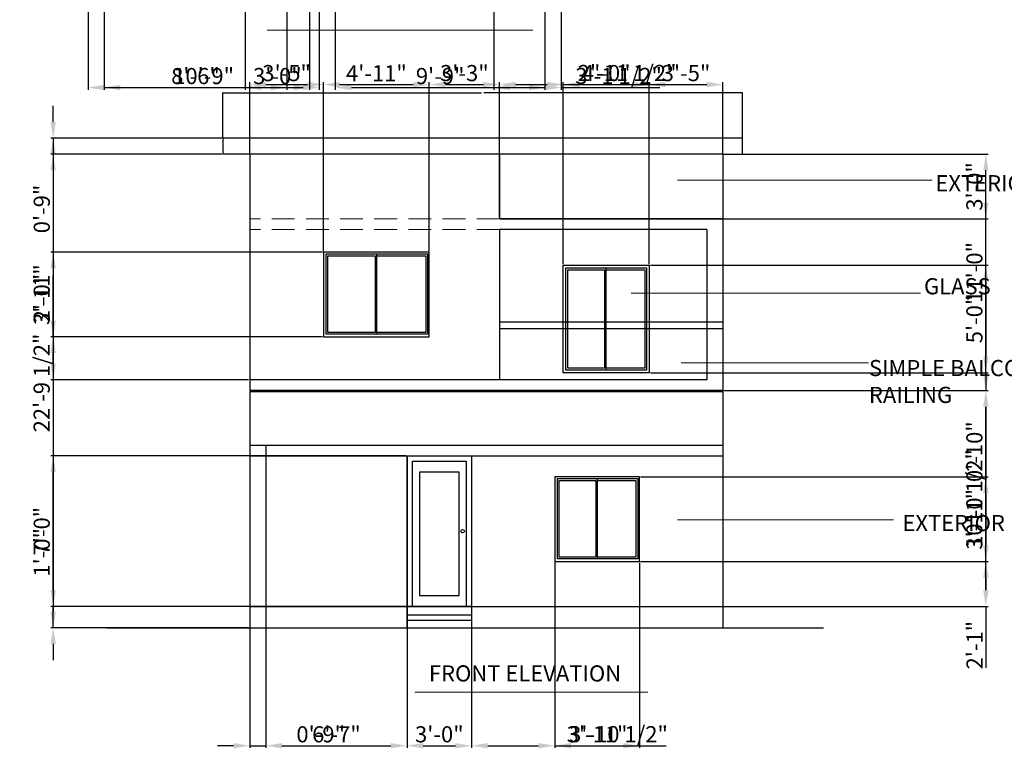
# Model space of a CAD drawing. Units: inches. Extents: x 2429 to 3343, y 1496 to 2530.
# Tile 1 of 7: x 2442 to 2991, y 1496 to 1910. Entities that reach past the tile are written whole.
import ezdxf

# ---------------------------------------------------------------- set-up
doc = ezdxf.new("R2010")
doc.units = ezdxf.units.IN
doc.linetypes.add('DASHED', pattern=[19.05, 12.7, -6.35])
for name, color, linetype, lineweight in [('A-ANNO-DIMS', 2, 'Continuous', 18), ('A-ANNO-TEXT', 7, 'Continuous', 18), ('A-ELEV', 7, 'Continuous', 25), ('A-ELEV-OVHD', 8, 'DASHED', 18)]:
    doc.layers.add(name, color=color, linetype=linetype, lineweight=lineweight)
doc.styles.get("Standard").update_dxf_attribs({"font": 'arial.ttf'})
doc.dimstyles.new('ISO-25', dxfattribs={"dimtxt": 9, "dimasz": 9, "dimexe": 1.25, "dimexo": 0.625, "dimtad": 1, "dimdec": 1, "dimlunit": 3, "dimtxsty": 'Standard', "dimcen": 9, "dimadec": 0, "dimazin": 0, "dimtfac": 1, "dimtdec": 1, "dimtmove": 0, "dimatfit": 3, "dimfxl": 1, "dimarcsym": 0})
doc.dimstyles.get("Standard").update_dxf_attribs({"dimtxt": 0.18, "dimasz": 0.18, "dimexe": 0.18, "dimexo": 0.0625, "dimgap": 0.09, "dimtad": 0, "dimtih": 1, "dimtoh": 1, "dimdec": 4, "dimzin": 0, "dimdsep": 46, "dimtxsty": 'Standard', "dimcen": 0.09, "dimadec": 0, "dimazin": 0, "dimtfac": 1, "dimtdec": 4, "dimtofl": 0, "dimtmove": 0, "dimatfit": 3, "dimfxl": 1, "dimtolj": 1, "dimtzin": 0, "dimarcsym": 0})

# ---------------------------------------------------------------- blocks, each defined once
blk = doc.blocks.new('*U18')
blk.add_lwpolyline([(3.12, 0.01), (0.12, 0.01), (0.12, 84.01), (36.12, 84.01), (36.12, 0.01), (33.12, 0.01)])
for points in [[(33.12, 80.99), (33.12, 0.01), (3.12, 0.01), (3.12, 80.99)], [(29.12, 6.01), (29.12, 74.99), (7.12, 74.99), (7.12, 6.01)]]:
    blk.add_lwpolyline(points, close=True)
blk.add_circle((31.12, 42.01), 1)
blk = doc.blocks.new('*U15')
for p, q in [((38.1, 38.1), (38.1, 1176.3)), ((38.1, 1176.3), (607.2, 1176.3)), ((607.2, 38.1), (607.2, 1176.3)), ((607.2, 1176.3), (1176.3, 1176.3)), ((1176.3, 1176.3), (1176.3, 38.1)), ((607.2, 38.1), (38.1, 38.1)), ((1176.3, 38.1), (607.2, 38.1))]:
    blk.add_line(p, q)
blk.add_lwpolyline([(0, 0), (1200, 0), (1200, 1200), (0, 1200)], close=True)
for points in [[(581.8, 1150.9), (581.8, 63.5), (63.5, 63.5), (63.5, 1150.9), (581.8, 1150.9)], [(607.2, 1150.9), (1150.9, 1150.9), (1150.9, 63.5), (607.2, 63.5)]]:
    blk.add_lwpolyline(points)
blk = doc.blocks.new('*U20')
for p, q in [((1.5, 1.5), (1.5, 58.5)), ((1.5, 58.5), (24, 58.5)), ((24, 1.5), (24, 58.5)), ((24, 58.5), (46.5, 58.5)), ((46.5, 58.5), (46.5, 1.5)), ((24, 1.5), (1.5, 1.5)), ((46.5, 1.5), (24, 1.5))]:
    blk.add_line(p, q)
blk.add_lwpolyline([(0, 0), (0, 60), (48, 60), (48, 0)], close=True)
for points in [[(23, 57.5), (23, 2.5), (2.5, 2.5), (2.5, 57.5), (23, 57.5)], [(24, 57.5), (45.5, 57.5), (45.5, 2.5), (24, 2.5)]]:
    blk.add_lwpolyline(points)
blk = doc.blocks.new('*U21')
for p, q in [((38.1, 38.1), (38.1, 1176.3)), ((38.1, 1176.3), (757.2, 1176.3)), ((757.2, 38.1), (757.2, 1176.3)), ((757.2, 1176.3), (1476.3, 1176.3)), ((1476.3, 1176.3), (1476.3, 38.1)), ((757.2, 38.1), (38.1, 38.1)), ((1476.3, 38.1), (757.2, 38.1))]:
    blk.add_line(p, q)
blk.add_lwpolyline([(0, 0), (1500, 0), (1500, 1200), (0, 1200)], close=True)
for points in [[(731.8, 1150.9), (731.8, 63.5), (63.5, 63.5), (63.5, 1150.9), (731.8, 1150.9)], [(757.2, 1150.9), (1450.9, 1150.9), (1450.9, 63.5), (757.2, 63.5)]]:
    blk.add_lwpolyline(points)
blk = doc.blocks.new('*D22')
at = {"layer": 'A-ANNO-DIMS', "color": 0, "lineweight": -2, "transparency": 16777216}
for p, q in [((2554.96, 1843.52), (2554.96, 1868.85)), ((2555.14, 1868.67), (2699.36, 1868.67)), ((2844.78, 1868.67), (2700.57, 1868.67)), ((2844.96, 1843.52), (2844.96, 1868.85))]:
    blk.add_line(p, q, dxfattribs=at)
at = {"layer": 'A-ANNO-DIMS', "color": 0, "transparency": 16777216}
for points in [[(2555.14, 1868.7), (2555.14, 1868.64), (2554.96, 1868.67)], [(2844.78, 1868.7), (2844.78, 1868.64), (2844.96, 1868.67)]]:
    blk.add_solid(points, dxfattribs=at)
at = {"layer": 'Defpoints', "color": 0, "transparency": 16777216}
for p in [(2844.96, 1868.67), (2554.96, 1843.46), (2844.96, 1843.46)]:
    blk.add_point(p, dxfattribs=at)
at = {"layer": 'A-ANNO-DIMS', "color": 0, "transparency": 16777216, "insert": (2699.96, 1868.67), "char_height": 0.18, "attachment_point": 5}
blk.add_mtext('\\A1;290.0000', dxfattribs=at)
blk = doc.blocks.new('*D34')
at = {"layer": 'A-ANNO-DIMS', "color": 0, "lineweight": -2, "transparency": 16777216}
for p, q in [((2590.68, 2320.13), (2590.68, 1870.45)), ((2488.77, 2248.13), (2488.77, 1870.45)), ((2497.77, 1871.7), (2581.68, 1871.7))]:
    blk.add_line(p, q, dxfattribs=at)
at = {"layer": 'A-ANNO-DIMS', "color": 0, "transparency": 16777216}
for points in [[(2497.77, 1873.2), (2497.77, 1870.2), (2488.77, 1871.7)], [(2581.68, 1873.2), (2581.68, 1870.2), (2590.68, 1871.7)]]:
    blk.add_solid(points, dxfattribs=at)
at = {"layer": 'Defpoints', "color": 0, "transparency": 16777216}
for p in [(2590.68, 2320.75), (2488.77, 2248.75), (2590.68, 1871.7)]:
    blk.add_point(p, dxfattribs=at)
at = {"layer": 'A-ANNO-DIMS', "color": 0, "transparency": 16777216, "insert": (2539.73, 1876.92), "char_height": 9, "attachment_point": 5}
blk.add_mtext('8\'-6"', dxfattribs=at)
blk = doc.blocks.new('*D38')
at = {"layer": 'A-ANNO-DIMS', "color": 0, "lineweight": -2, "transparency": 16777216}
for p, q in [((2617.77, 2011.13), (2617.77, 1870.45)), ((2734.77, 2011.13), (2734.77, 1870.45)), ((2626.77, 1871.7), (2725.77, 1871.7))]:
    blk.add_line(p, q, dxfattribs=at)
at = {"layer": 'A-ANNO-DIMS', "color": 0, "transparency": 16777216}
for points in [[(2626.77, 1873.2), (2626.77, 1870.2), (2617.77, 1871.7)], [(2725.77, 1873.2), (2725.77, 1870.2), (2734.77, 1871.7)]]:
    blk.add_solid(points, dxfattribs=at)
at = {"layer": 'Defpoints', "color": 0, "transparency": 16777216}
for p in [(2617.77, 2011.75), (2734.77, 2011.75), (2734.77, 1871.7)]:
    blk.add_point(p, dxfattribs=at)
at = {"layer": 'A-ANNO-DIMS', "color": 0, "transparency": 16777216, "insert": (2676.27, 1876.92), "char_height": 9, "attachment_point": 5}
blk.add_mtext('9\'-9"', dxfattribs=at)
blk = doc.blocks.new('*D44')
at = {"layer": 'A-ANNO-DIMS', "color": 0, "lineweight": -2, "transparency": 16777216}
for p, q in [((2608.77, 2002.13), (2608.77, 1870.45)), ((2479.77, 1970.81), (2479.77, 1870.45)), ((2488.77, 1871.7), (2599.77, 1871.7))]:
    blk.add_line(p, q, dxfattribs=at)
at = {"layer": 'A-ANNO-DIMS', "color": 0, "transparency": 16777216}
for points in [[(2488.77, 1873.2), (2488.77, 1870.2), (2479.77, 1871.7)], [(2599.77, 1873.2), (2599.77, 1870.2), (2608.77, 1871.7)]]:
    blk.add_solid(points, dxfattribs=at)
at = {"layer": 'Defpoints', "color": 0, "transparency": 16777216}
for p in [(2608.77, 2002.75), (2479.77, 1971.44), (2608.77, 1871.7)]:
    blk.add_point(p, dxfattribs=at)
at = {"layer": 'A-ANNO-DIMS', "color": 0, "transparency": 16777216, "insert": (2544.27, 1876.92), "char_height": 9, "attachment_point": 5}
blk.add_mtext('10\'-9"', dxfattribs=at)
blk = doc.blocks.new('*D45')
at = {"layer": 'A-ANNO-DIMS', "color": 0, "lineweight": -2, "transparency": 16777216}
for p, q in [((2567.44, 2072.42), (2567.44, 1870.45)), ((2603.44, 2071.13), (2603.44, 1870.45)), ((2576.44, 1871.7), (2594.44, 1871.7))]:
    blk.add_line(p, q, dxfattribs=at)
at = {"layer": 'A-ANNO-DIMS', "color": 0, "transparency": 16777216}
for points in [[(2576.44, 1873.2), (2576.44, 1870.2), (2567.44, 1871.7)], [(2594.44, 1873.2), (2594.44, 1870.2), (2603.44, 1871.7)]]:
    blk.add_solid(points, dxfattribs=at)
at = {"layer": 'Defpoints', "color": 0, "transparency": 16777216}
for p in [(2567.44, 2073.04), (2603.44, 2071.75), (2603.44, 1871.7)]:
    blk.add_point(p, dxfattribs=at)
at = {"layer": 'A-ANNO-DIMS', "color": 0, "transparency": 16777216, "insert": (2585.44, 1876.92), "char_height": 9, "attachment_point": 5}
blk.add_mtext('3\'-0"', dxfattribs=at)
blk = doc.blocks.new('*D55')
at = {"layer": 'A-ANNO-DIMS', "color": 0, "lineweight": -2, "transparency": 16777216}
for p, q in [((2706.27, 2002.13), (2706.27, 1870.45)), ((2743.77, 2002.13), (2743.77, 1870.45)), ((2715.27, 1871.7), (2734.77, 1871.7)), ((2743.77, 1871.7), (2798.91, 1871.7))]:
    blk.add_line(p, q, dxfattribs=at)
at = {"layer": 'A-ANNO-DIMS', "color": 0, "transparency": 16777216}
for points in [[(2715.27, 1873.2), (2715.27, 1870.2), (2706.27, 1871.7)], [(2734.77, 1873.2), (2734.77, 1870.2), (2743.77, 1871.7)]]:
    blk.add_solid(points, dxfattribs=at)
at = {"layer": 'Defpoints', "color": 0, "transparency": 16777216}
for p in [(2706.27, 2002.75), (2743.77, 2002.75), (2743.77, 1871.7)]:
    blk.add_point(p, dxfattribs=at)
at = {"layer": 'A-ANNO-DIMS', "color": 0, "transparency": 16777216, "insert": (2775.84, 1876.98), "char_height": 9, "attachment_point": 5}
blk.add_mtext('3\'-1 1/2"', dxfattribs=at)
blk = doc.blocks.new('*D84')
at = {"layer": 'A-ANNO-DIMS', "color": 0, "lineweight": -2, "transparency": 16777216}
for p, q in [((2554.34, 1843.46), (2459.08, 1843.46)), ((2460.33, 1834.46), (2460.33, 1579)), ((2569.38, 1570), (2459.08, 1570))]:
    blk.add_line(p, q, dxfattribs=at)
at = {"layer": 'A-ANNO-DIMS', "color": 0, "transparency": 16777216}
for points in [[(2458.83, 1834.46), (2461.83, 1834.46), (2460.33, 1843.46)], [(2458.83, 1579), (2461.83, 1579), (2460.33, 1570)]]:
    blk.add_solid(points, dxfattribs=at)
at = {"layer": 'Defpoints', "color": 0, "transparency": 16777216}
for p in [(2554.96, 1843.46), (2460.33, 1570), (2570, 1570)]:
    blk.add_point(p, dxfattribs=at)
at = {"layer": 'A-ANNO-DIMS', "color": 0, "transparency": 16777216, "insert": (2455.05, 1706.73), "char_height": 9, "attachment_point": 5, "rotation": 90}
blk.add_mtext('22\'-9 1/2"', dxfattribs=at)
blk = doc.blocks.new('*D85')
at = {"layer": 'A-ANNO-DIMS', "color": 0, "lineweight": -2, "transparency": 16777216}
for p, q in [((2460.33, 1852.46), (2460.33, 1861.46)), ((2554.34, 1843.46), (2459.08, 1843.46)), ((2460.33, 1843.46), (2460.33, 1834.46)), ((2554.34, 1834.46), (2459.08, 1834.46)), ((2460.33, 1825.46), (2460.33, 1791.28))]:
    blk.add_line(p, q, dxfattribs=at)
at = {"layer": 'A-ANNO-DIMS', "color": 0, "transparency": 16777216}
for points in [[(2458.83, 1852.46), (2461.83, 1852.46), (2460.33, 1843.46)], [(2458.83, 1825.46), (2461.83, 1825.46), (2460.33, 1834.46)]]:
    blk.add_solid(points, dxfattribs=at)
at = {"layer": 'Defpoints', "color": 0, "transparency": 16777216}
for p in [(2554.96, 1843.46), (2460.33, 1834.46), (2554.96, 1834.46)]:
    blk.add_point(p, dxfattribs=at)
at = {"layer": 'A-ANNO-DIMS', "color": 0, "transparency": 16777216, "insert": (2455.11, 1803.87), "char_height": 9, "attachment_point": 5, "rotation": 90}
blk.add_mtext('0\'-9"', dxfattribs=at)
blk = doc.blocks.new('*D86')
at = {"layer": 'A-ANNO-DIMS', "color": 0, "lineweight": -2, "transparency": 16777216}
for p, q in [((2460.33, 1591), (2460.33, 1624.33)), ((2569.38, 1582), (2459.08, 1582)), ((2460.33, 1570), (2460.33, 1582)), ((2569.38, 1570), (2459.08, 1570)), ((2460.33, 1561), (2460.33, 1552))]:
    blk.add_line(p, q, dxfattribs=at)
at = {"layer": 'A-ANNO-DIMS', "color": 0, "transparency": 16777216}
for points in [[(2458.83, 1591), (2461.83, 1591), (2460.33, 1582)], [(2458.83, 1561), (2461.83, 1561), (2460.33, 1570)]]:
    blk.add_solid(points, dxfattribs=at)
at = {"layer": 'Defpoints', "color": 0, "transparency": 16777216}
for p in [(2460.33, 1582), (2570, 1582), (2570, 1570)]:
    blk.add_point(p, dxfattribs=at)
at = {"layer": 'A-ANNO-DIMS', "color": 0, "transparency": 16777216, "insert": (2455.11, 1612.16), "char_height": 9, "attachment_point": 5, "rotation": 90}
blk.add_mtext('1\'-0"', dxfattribs=at)
blk = doc.blocks.new('*D87')
at = {"layer": 'A-ANNO-DIMS', "color": 0, "lineweight": -2, "transparency": 16777216}
for p, q in [((2834.63, 1702.46), (2982.04, 1702.46)), ((2980.79, 1591), (2980.79, 1693.46)), ((2834.63, 1582), (2982.04, 1582))]:
    blk.add_line(p, q, dxfattribs=at)
at = {"layer": 'A-ANNO-DIMS', "color": 0, "transparency": 16777216}
for points in [[(2979.29, 1693.46), (2982.29, 1693.46), (2980.79, 1702.46)], [(2979.29, 1591), (2982.29, 1591), (2980.79, 1582)]]:
    blk.add_solid(points, dxfattribs=at)
at = {"layer": 'Defpoints', "color": 0, "transparency": 16777216}
for p in [(2834.01, 1702.46), (2980.79, 1702.46), (2834, 1582)]:
    blk.add_point(p, dxfattribs=at)
at = {"layer": 'A-ANNO-DIMS', "color": 0, "transparency": 16777216, "insert": (2975.51, 1642.23), "char_height": 9, "attachment_point": 5, "rotation": 90}
blk.add_mtext('10\'-0 1/2"', dxfattribs=at)
blk = doc.blocks.new('*D88')
at = {"layer": 'A-ANNO-DIMS', "color": 0, "lineweight": -2, "transparency": 16777216}
for p, q in [((2834.63, 1834.46), (2982.04, 1834.46)), ((2980.79, 1711.46), (2980.79, 1825.46)), ((2834.63, 1702.46), (2982.04, 1702.46))]:
    blk.add_line(p, q, dxfattribs=at)
at = {"layer": 'A-ANNO-DIMS', "color": 0, "transparency": 16777216}
for points in [[(2979.29, 1825.46), (2982.29, 1825.46), (2980.79, 1834.46)], [(2979.29, 1711.46), (2982.29, 1711.46), (2980.79, 1702.46)]]:
    blk.add_solid(points, dxfattribs=at)
at = {"layer": 'Defpoints', "color": 0, "transparency": 16777216}
for p in [(2834.01, 1834.46), (2980.79, 1834.46), (2834.01, 1702.46)]:
    blk.add_point(p, dxfattribs=at)
at = {"layer": 'A-ANNO-DIMS', "color": 0, "transparency": 16777216, "insert": (2975.57, 1768.46), "char_height": 9, "attachment_point": 5, "rotation": 90}
blk.add_mtext('11\'-0"', dxfattribs=at)
blk = doc.blocks.new('*D89')
at = {"layer": 'A-ANNO-DIMS', "color": 0, "lineweight": -2, "transparency": 16777216}
for p, q in [((2570.01, 1835.08), (2570.01, 1874.61)), ((2611.16, 1780.33), (2611.16, 1874.61)), ((2579.01, 1873.36), (2602.16, 1873.36))]:
    blk.add_line(p, q, dxfattribs=at)
at = {"layer": 'A-ANNO-DIMS', "color": 0, "transparency": 16777216}
for points in [[(2579.01, 1874.86), (2579.01, 1871.86), (2570.01, 1873.36)], [(2602.16, 1874.86), (2602.16, 1871.86), (2611.16, 1873.36)]]:
    blk.add_solid(points, dxfattribs=at)
at = {"layer": 'Defpoints', "color": 0, "transparency": 16777216}
for p in [(2611.16, 1873.36), (2570.01, 1834.46), (2611.16, 1779.7)]:
    blk.add_point(p, dxfattribs=at)
at = {"layer": 'A-ANNO-DIMS', "color": 0, "transparency": 16777216, "insert": (2590.58, 1878.58), "char_height": 9, "attachment_point": 5}
blk.add_mtext('3\'-5"', dxfattribs=at)
blk = doc.blocks.new('*D90')
at = {"layer": 'A-ANNO-DIMS', "color": 0, "lineweight": -2, "transparency": 16777216}
for p, q in [((2611.16, 1780.33), (2611.16, 1874.61)), ((2670.21, 1780.33), (2670.21, 1874.61)), ((2620.16, 1873.36), (2661.21, 1873.36))]:
    blk.add_line(p, q, dxfattribs=at)
at = {"layer": 'A-ANNO-DIMS', "color": 0, "transparency": 16777216}
for points in [[(2620.16, 1874.86), (2620.16, 1871.86), (2611.16, 1873.36)], [(2661.21, 1874.86), (2661.21, 1871.86), (2670.21, 1873.36)]]:
    blk.add_solid(points, dxfattribs=at)
at = {"layer": 'Defpoints', "color": 0, "transparency": 16777216}
for p in [(2670.21, 1873.36), (2611.16, 1779.7), (2670.21, 1779.7)]:
    blk.add_point(p, dxfattribs=at)
at = {"layer": 'A-ANNO-DIMS', "color": 0, "transparency": 16777216, "insert": (2640.69, 1878.5), "char_height": 9, "attachment_point": 5}
blk.add_mtext('4\'-11"', dxfattribs=at)
blk = doc.blocks.new('*D91')
at = {"layer": 'A-ANNO-DIMS', "color": 0, "lineweight": -2, "transparency": 16777216}
for p, q in [((2670.21, 1780.33), (2670.21, 1874.61)), ((2709.37, 1799.08), (2709.37, 1874.61)), ((2679.21, 1873.36), (2700.37, 1873.36))]:
    blk.add_line(p, q, dxfattribs=at)
at = {"layer": 'A-ANNO-DIMS', "color": 0, "transparency": 16777216}
for points in [[(2679.21, 1874.86), (2679.21, 1871.86), (2670.21, 1873.36)], [(2700.37, 1874.86), (2700.37, 1871.86), (2709.37, 1873.36)]]:
    blk.add_solid(points, dxfattribs=at)
at = {"layer": 'Defpoints', "color": 0, "transparency": 16777216}
for p in [(2709.37, 1873.36), (2709.37, 1798.46), (2670.21, 1779.7)]:
    blk.add_point(p, dxfattribs=at)
at = {"layer": 'A-ANNO-DIMS', "color": 0, "transparency": 16777216, "insert": (2689.79, 1878.58), "char_height": 9, "attachment_point": 5}
blk.add_mtext('3\'-3"', dxfattribs=at)
blk = doc.blocks.new('*D92')
at = {"layer": 'A-ANNO-DIMS', "color": 0, "lineweight": -2, "transparency": 16777216}
for p, q in [((2709.37, 1799.08), (2709.37, 1874.61)), ((2744.96, 1773.08), (2744.96, 1874.61)), ((2718.37, 1873.36), (2735.96, 1873.36)), ((2744.96, 1873.36), (2807.25, 1873.36))]:
    blk.add_line(p, q, dxfattribs=at)
at = {"layer": 'A-ANNO-DIMS', "color": 0, "transparency": 16777216}
for points in [[(2718.37, 1874.86), (2718.37, 1871.86), (2709.37, 1873.36)], [(2735.96, 1874.86), (2735.96, 1871.86), (2744.96, 1873.36)]]:
    blk.add_solid(points, dxfattribs=at)
at = {"layer": 'Defpoints', "color": 0, "transparency": 16777216}
for p in [(2744.96, 1873.36), (2709.37, 1798.46), (2744.96, 1772.46)]:
    blk.add_point(p, dxfattribs=at)
at = {"layer": 'A-ANNO-DIMS', "color": 0, "transparency": 16777216, "insert": (2780.61, 1878.64), "char_height": 9, "attachment_point": 5}
blk.add_mtext('2\'-11 1/2"', dxfattribs=at)
blk = doc.blocks.new('*D93')
at = {"layer": 'A-ANNO-DIMS', "color": 0, "lineweight": -2, "transparency": 16777216}
for p, q in [((2744.96, 1773.08), (2744.96, 1874.61)), ((2792.96, 1773.08), (2792.96, 1874.61)), ((2753.96, 1873.36), (2783.96, 1873.36))]:
    blk.add_line(p, q, dxfattribs=at)
at = {"layer": 'A-ANNO-DIMS', "color": 0, "transparency": 16777216}
for points in [[(2753.96, 1874.86), (2753.96, 1871.86), (2744.96, 1873.36)], [(2783.96, 1874.86), (2783.96, 1871.86), (2792.96, 1873.36)]]:
    blk.add_solid(points, dxfattribs=at)
at = {"layer": 'Defpoints', "color": 0, "transparency": 16777216}
for p in [(2792.96, 1873.36), (2744.96, 1772.46), (2792.96, 1772.46)]:
    blk.add_point(p, dxfattribs=at)
at = {"layer": 'A-ANNO-DIMS', "color": 0, "transparency": 16777216, "insert": (2768.96, 1878.58), "char_height": 9, "attachment_point": 5}
blk.add_mtext('4\'-0"', dxfattribs=at)
blk = doc.blocks.new('*D94')
at = {"layer": 'A-ANNO-DIMS', "color": 0, "lineweight": -2, "transparency": 16777216}
for p, q in [((2792.96, 1773.08), (2792.96, 1874.61)), ((2834.01, 1835.08), (2834.01, 1874.61)), ((2801.96, 1873.36), (2825.01, 1873.36))]:
    blk.add_line(p, q, dxfattribs=at)
at = {"layer": 'A-ANNO-DIMS', "color": 0, "transparency": 16777216}
for points in [[(2801.96, 1874.86), (2801.96, 1871.86), (2792.96, 1873.36)], [(2825.01, 1874.86), (2825.01, 1871.86), (2834.01, 1873.36)]]:
    blk.add_solid(points, dxfattribs=at)
at = {"layer": 'Defpoints', "color": 0, "transparency": 16777216}
for p in [(2834.01, 1873.36), (2834.01, 1834.46), (2792.96, 1772.46)]:
    blk.add_point(p, dxfattribs=at)
at = {"layer": 'A-ANNO-DIMS', "color": 0, "transparency": 16777216, "insert": (2813.48, 1878.58), "char_height": 9, "attachment_point": 5}
blk.add_mtext('3\'-5"', dxfattribs=at)
blk = doc.blocks.new('*D95')
at = {"layer": 'A-ANNO-DIMS', "color": 0, "lineweight": -2, "transparency": 16777216}
for p, q in [((2579, 1671.38), (2579, 1502.93)), ((2657.8, 1665.38), (2657.8, 1502.93)), ((2588, 1504.18), (2648.8, 1504.18))]:
    blk.add_line(p, q, dxfattribs=at)
at = {"layer": 'A-ANNO-DIMS', "color": 0, "transparency": 16777216}
for points in [[(2588, 1505.68), (2588, 1502.68), (2579, 1504.18)], [(2648.8, 1505.68), (2648.8, 1502.68), (2657.8, 1504.18)]]:
    blk.add_solid(points, dxfattribs=at)
at = {"layer": 'Defpoints', "color": 0, "transparency": 16777216}
for p in [(2579, 1672), (2657.8, 1666), (2657.8, 1504.18)]:
    blk.add_point(p, dxfattribs=at)
at = {"layer": 'A-ANNO-DIMS', "color": 0, "transparency": 16777216, "insert": (2618.4, 1509.4), "char_height": 9, "attachment_point": 5}
blk.add_mtext('6\'-7"', dxfattribs=at)
blk = doc.blocks.new('*D96')
at = {"layer": 'A-ANNO-DIMS', "color": 0, "lineweight": -2, "transparency": 16777216}
for p, q in [((2570, 1671.38), (2570, 1502.93)), ((2579, 1671.38), (2579, 1502.93)), ((2561, 1504.18), (2552, 1504.18)), ((2570, 1504.18), (2579, 1504.18)), ((2588, 1504.18), (2622.17, 1504.18))]:
    blk.add_line(p, q, dxfattribs=at)
at = {"layer": 'A-ANNO-DIMS', "color": 0, "transparency": 16777216}
for points in [[(2561, 1505.68), (2561, 1502.68), (2570, 1504.18)], [(2588, 1505.68), (2588, 1502.68), (2579, 1504.18)]]:
    blk.add_solid(points, dxfattribs=at)
at = {"layer": 'Defpoints', "color": 0, "transparency": 16777216}
for p in [(2570, 1672), (2579, 1672), (2579, 1504.18)]:
    blk.add_point(p, dxfattribs=at)
at = {"layer": 'A-ANNO-DIMS', "color": 0, "transparency": 16777216, "insert": (2609.59, 1509.4), "char_height": 9, "attachment_point": 5}
blk.add_mtext('0\'-9"', dxfattribs=at)
blk = doc.blocks.new('*D97')
at = {"layer": 'A-ANNO-DIMS', "color": 0, "lineweight": -2, "transparency": 16777216}
for p, q in [((2657.8, 1581.38), (2657.8, 1502.93)), ((2693.8, 1581.38), (2693.8, 1502.93)), ((2666.8, 1504.18), (2684.8, 1504.18))]:
    blk.add_line(p, q, dxfattribs=at)
at = {"layer": 'A-ANNO-DIMS', "color": 0, "transparency": 16777216}
for points in [[(2666.8, 1505.68), (2666.8, 1502.68), (2657.8, 1504.18)], [(2684.8, 1505.68), (2684.8, 1502.68), (2693.8, 1504.18)]]:
    blk.add_solid(points, dxfattribs=at)
at = {"layer": 'Defpoints', "color": 0, "transparency": 16777216}
for p in [(2657.8, 1582), (2693.8, 1582), (2693.8, 1504.18)]:
    blk.add_point(p, dxfattribs=at)
at = {"layer": 'A-ANNO-DIMS', "color": 0, "transparency": 16777216, "insert": (2675.8, 1509.4), "char_height": 9, "attachment_point": 5}
blk.add_mtext('3\'-0"', dxfattribs=at)
blk = doc.blocks.new('*D98')
at = {"layer": 'A-ANNO-DIMS', "color": 0, "lineweight": -2, "transparency": 16777216}
for p, q in [((2693.8, 1665.38), (2693.8, 1502.93)), ((2740.23, 1653.63), (2740.23, 1502.93)), ((2702.8, 1504.18), (2731.23, 1504.18)), ((2740.23, 1504.18), (2802.36, 1504.18))]:
    blk.add_line(p, q, dxfattribs=at)
at = {"layer": 'A-ANNO-DIMS', "color": 0, "transparency": 16777216}
for points in [[(2702.8, 1505.68), (2702.8, 1502.68), (2693.8, 1504.18)], [(2731.23, 1505.68), (2731.23, 1502.68), (2740.23, 1504.18)]]:
    blk.add_solid(points, dxfattribs=at)
at = {"layer": 'Defpoints', "color": 0, "transparency": 16777216}
for p in [(2693.8, 1666), (2740.23, 1654.26), (2740.23, 1504.18)]:
    blk.add_point(p, dxfattribs=at)
at = {"layer": 'A-ANNO-DIMS', "color": 0, "transparency": 16777216, "insert": (2775.79, 1509.46), "char_height": 9, "attachment_point": 5}
blk.add_mtext('3\'-10 1/2"', dxfattribs=at)
blk = doc.blocks.new('*D99')
at = {"layer": 'A-ANNO-DIMS', "color": 0, "lineweight": -2, "transparency": 16777216}
for p, q in [((2740.23, 1606.39), (2740.23, 1502.93)), ((2787.47, 1606.39), (2787.47, 1502.93)), ((2749.23, 1504.18), (2778.47, 1504.18))]:
    blk.add_line(p, q, dxfattribs=at)
at = {"layer": 'A-ANNO-DIMS', "color": 0, "transparency": 16777216}
for points in [[(2749.23, 1505.68), (2749.23, 1502.68), (2740.23, 1504.18)], [(2778.47, 1505.68), (2778.47, 1502.68), (2787.47, 1504.18)]]:
    blk.add_solid(points, dxfattribs=at)
at = {"layer": 'Defpoints', "color": 0, "transparency": 16777216}
for p in [(2740.23, 1607.01), (2787.47, 1607.01), (2787.47, 1504.18)]:
    blk.add_point(p, dxfattribs=at)
at = {"layer": 'A-ANNO-DIMS', "color": 0, "transparency": 16777216, "insert": (2763.85, 1509.4), "char_height": 9, "attachment_point": 5}
blk.add_mtext('3\'-11"', dxfattribs=at)
blk = doc.blocks.new('*D100')
at = {"layer": 'A-ANNO-DIMS', "color": 0, "lineweight": -2, "transparency": 16777216}
for p, q in [((2657.17, 1666), (2459.08, 1666)), ((2460.33, 1591), (2460.33, 1657)), ((2657.17, 1582), (2459.08, 1582))]:
    blk.add_line(p, q, dxfattribs=at)
at = {"layer": 'A-ANNO-DIMS', "color": 0, "transparency": 16777216}
for points in [[(2458.83, 1657), (2461.83, 1657), (2460.33, 1666)], [(2458.83, 1591), (2461.83, 1591), (2460.33, 1582)]]:
    blk.add_solid(points, dxfattribs=at)
at = {"layer": 'Defpoints', "color": 0, "transparency": 16777216}
for p in [(2460.33, 1666), (2657.8, 1666), (2657.8, 1582)]:
    blk.add_point(p, dxfattribs=at)
at = {"layer": 'A-ANNO-DIMS', "color": 0, "transparency": 16777216, "insert": (2455.11, 1624), "char_height": 9, "attachment_point": 5, "rotation": 90}
blk.add_mtext('7\'-0"', dxfattribs=at)
blk = doc.blocks.new('*D101')
at = {"layer": 'A-ANNO-DIMS', "color": 0, "lineweight": -2, "transparency": 16777216}
for p, q in [((2788.1, 1654.26), (2982.04, 1654.26)), ((2980.79, 1645.26), (2980.79, 1616.01)), ((2788.1, 1607.01), (2982.04, 1607.01))]:
    blk.add_line(p, q, dxfattribs=at)
at = {"layer": 'A-ANNO-DIMS', "color": 0, "transparency": 16777216}
for points in [[(2979.29, 1645.26), (2982.29, 1645.26), (2980.79, 1654.26)], [(2979.29, 1616.01), (2982.29, 1616.01), (2980.79, 1607.01)]]:
    blk.add_solid(points, dxfattribs=at)
at = {"layer": 'Defpoints', "color": 0, "transparency": 16777216}
for p in [(2787.47, 1654.26), (2787.47, 1607.01), (2980.79, 1607.01)]:
    blk.add_point(p, dxfattribs=at)
at = {"layer": 'A-ANNO-DIMS', "color": 0, "transparency": 16777216, "insert": (2975.57, 1630.63), "char_height": 9, "attachment_point": 5, "rotation": 90}
blk.add_mtext('3\'-11"', dxfattribs=at)
blk = doc.blocks.new('*D102')
at = {"layer": 'A-ANNO-DIMS', "color": 0, "lineweight": -2, "transparency": 16777216}
for p, q in [((2788.1, 1607.01), (2982.04, 1607.01)), ((2980.79, 1598.01), (2980.79, 1591)), ((2834.63, 1582), (2982.04, 1582)), ((2980.79, 1582), (2980.79, 1547.67))]:
    blk.add_line(p, q, dxfattribs=at)
at = {"layer": 'A-ANNO-DIMS', "color": 0, "transparency": 16777216}
for points in [[(2979.29, 1598.01), (2982.29, 1598.01), (2980.79, 1607.01)], [(2979.29, 1591), (2982.29, 1591), (2980.79, 1582)]]:
    blk.add_solid(points, dxfattribs=at)
at = {"layer": 'Defpoints', "color": 0, "transparency": 16777216}
for p in [(2787.47, 1607.01), (2834, 1582), (2980.79, 1582)]:
    blk.add_point(p, dxfattribs=at)
at = {"layer": 'A-ANNO-DIMS', "color": 0, "transparency": 16777216, "insert": (2975.65, 1560.34), "char_height": 9, "attachment_point": 5, "rotation": 90}
blk.add_mtext('2\'-1"', dxfattribs=at)
blk = doc.blocks.new('*D103')
at = {"layer": 'A-ANNO-DIMS', "color": 0, "lineweight": -2, "transparency": 16777216}
for p, q in [((2610.53, 1779.7), (2459.08, 1779.7)), ((2460.33, 1770.7), (2460.33, 1741.46)), ((2610.53, 1732.46), (2459.08, 1732.46))]:
    blk.add_line(p, q, dxfattribs=at)
at = {"layer": 'A-ANNO-DIMS', "color": 0, "transparency": 16777216}
for points in [[(2458.83, 1770.7), (2461.83, 1770.7), (2460.33, 1779.7)], [(2458.83, 1741.46), (2461.83, 1741.46), (2460.33, 1732.46)]]:
    blk.add_solid(points, dxfattribs=at)
at = {"layer": 'Defpoints', "color": 0, "transparency": 16777216}
for p in [(2611.16, 1779.7), (2460.33, 1732.46), (2611.16, 1732.46)]:
    blk.add_point(p, dxfattribs=at)
at = {"layer": 'A-ANNO-DIMS', "color": 0, "transparency": 16777216, "insert": (2455.1, 1756.08), "char_height": 9, "attachment_point": 5, "rotation": 90}
blk.add_mtext('3\'-11"', dxfattribs=at)
blk = doc.blocks.new('*D104')
at = {"layer": 'A-ANNO-DIMS', "color": 0, "lineweight": -2, "transparency": 16777216}
for p, q in [((2460.33, 1732.46), (2460.33, 1766.78)), ((2610.53, 1732.46), (2459.08, 1732.46)), ((2460.33, 1717.46), (2460.33, 1723.46)), ((2569.38, 1708.46), (2459.08, 1708.46))]:
    blk.add_line(p, q, dxfattribs=at)
at = {"layer": 'A-ANNO-DIMS', "color": 0, "transparency": 16777216}
for points in [[(2458.83, 1723.46), (2461.83, 1723.46), (2460.33, 1732.46)], [(2458.83, 1717.46), (2461.83, 1717.46), (2460.33, 1708.46)]]:
    blk.add_solid(points, dxfattribs=at)
at = {"layer": 'Defpoints', "color": 0, "transparency": 16777216}
for p in [(2460.33, 1732.46), (2611.16, 1732.46), (2570.01, 1708.46)]:
    blk.add_point(p, dxfattribs=at)
at = {"layer": 'A-ANNO-DIMS', "color": 0, "transparency": 16777216, "insert": (2455.11, 1754.12), "char_height": 9, "attachment_point": 5, "rotation": 90}
blk.add_mtext('2\'-0"', dxfattribs=at)
blk = doc.blocks.new('*D105')
at = {"layer": 'A-ANNO-DIMS', "color": 0, "lineweight": -2, "transparency": 16777216}
for p, q in [((2793.59, 1772.46), (2982.04, 1772.46)), ((2980.79, 1763.46), (2980.79, 1721.46)), ((2793.59, 1712.46), (2982.04, 1712.46))]:
    blk.add_line(p, q, dxfattribs=at)
at = {"layer": 'A-ANNO-DIMS', "color": 0, "transparency": 16777216}
for points in [[(2979.29, 1763.46), (2982.29, 1763.46), (2980.79, 1772.46)], [(2979.29, 1721.46), (2982.29, 1721.46), (2980.79, 1712.46)]]:
    blk.add_solid(points, dxfattribs=at)
at = {"layer": 'Defpoints', "color": 0, "transparency": 16777216}
for p in [(2792.96, 1772.46), (2792.96, 1712.46), (2980.79, 1712.46)]:
    blk.add_point(p, dxfattribs=at)
at = {"layer": 'A-ANNO-DIMS', "color": 0, "transparency": 16777216, "insert": (2975.57, 1742.46), "char_height": 9, "attachment_point": 5, "rotation": 90}
blk.add_mtext('5\'-0"', dxfattribs=at)
blk = doc.blocks.new('*D106')
at = {"layer": 'A-ANNO-DIMS', "color": 0, "lineweight": -2, "transparency": 16777216}
for p, q in [((2980.79, 1721.46), (2980.79, 1730.46)), ((2793.59, 1712.46), (2982.04, 1712.46)), ((2980.79, 1712.46), (2980.79, 1702.46)), ((2834.63, 1702.46), (2982.04, 1702.46)), ((2980.79, 1693.46), (2980.79, 1652.29))]:
    blk.add_line(p, q, dxfattribs=at)
at = {"layer": 'A-ANNO-DIMS', "color": 0, "transparency": 16777216}
for points in [[(2979.29, 1721.46), (2982.29, 1721.46), (2980.79, 1712.46)], [(2979.29, 1693.46), (2982.29, 1693.46), (2980.79, 1702.46)]]:
    blk.add_solid(points, dxfattribs=at)
at = {"layer": 'Defpoints', "color": 0, "transparency": 16777216}
for p in [(2792.96, 1712.46), (2834.01, 1702.46), (2980.79, 1702.46)]:
    blk.add_point(p, dxfattribs=at)
at = {"layer": 'A-ANNO-DIMS', "color": 0, "transparency": 16777216, "insert": (2975.57, 1668.37), "char_height": 9, "attachment_point": 5, "rotation": 90}
blk.add_mtext('0\'-10"', dxfattribs=at)
blk = doc.blocks.new('*D107')
at = {"layer": 'A-ANNO-DIMS', "color": 0, "lineweight": -2, "transparency": 16777216}
for p, q in [((2834.63, 1834.46), (2982.04, 1834.46)), ((2980.79, 1807.46), (2980.79, 1825.46)), ((2710, 1798.46), (2982.04, 1798.46))]:
    blk.add_line(p, q, dxfattribs=at)
at = {"layer": 'A-ANNO-DIMS', "color": 0, "transparency": 16777216}
for points in [[(2979.29, 1825.46), (2982.29, 1825.46), (2980.79, 1834.46)], [(2979.29, 1807.46), (2982.29, 1807.46), (2980.79, 1798.46)]]:
    blk.add_solid(points, dxfattribs=at)
at = {"layer": 'Defpoints', "color": 0, "transparency": 16777216}
for p in [(2834.01, 1834.46), (2980.79, 1834.46), (2709.37, 1798.46)]:
    blk.add_point(p, dxfattribs=at)
at = {"layer": 'A-ANNO-DIMS', "color": 0, "transparency": 16777216, "insert": (2975.57, 1816.46), "char_height": 9, "attachment_point": 5, "rotation": 90}
blk.add_mtext('3\'-0"', dxfattribs=at)

msp = doc.modelspace()

# ---------------------------------------------------------------- linework, layer by layer
at = {"layer": 'A-ANNO-TEXT'}
for p, q in [((2579.72182, 1903.69967), (2727.973, 1903.69967)), ((2808.72605, 1819.93176), (2950.89229, 1819.93176)), ((2782.86988, 1756.92133), (2944.25417, 1756.92133)), ((2810.81431, 1717.98399), (2915.27116, 1717.98399)), ((2808.72547, 1630.25069), (2929.31783, 1630.25069)), ((2662.13382, 1534.07687), (2792.13018, 1534.07687))]:
    msp.add_line(p, q, dxfattribs=at)
at = {"layer": 'A-ELEV'}
for p, q in [((2844.96075, 1843.45698), (2554.96075, 1843.45698)), ((2554.96075, 1843.45698), (2554.96075, 1834.45698)), ((2844.96075, 1843.45698), (2554.96075, 1843.45698)), ((2554.96075, 1843.45698), (2554.96075, 1834.45698)), ((2844.96075, 1843.45698), (2554.96075, 1843.45698)), ((2554.96075, 1843.45698), (2554.96075, 1834.45698)), ((2844.96075, 1834.45698), (2844.96075, 1843.45698)), ((2844.96075, 1834.45698), (2844.96075, 1843.45698)), ((2844.96075, 1834.45698), (2844.96075, 1843.45698)), ((2834.00915, 1834.45698), (2554.96075, 1834.45698)), ((2834.00915, 1834.45698), (2554.96075, 1834.45698)), ((2834.00915, 1834.45698), (2554.96075, 1834.45698)), ((2570.00915, 1834.45698), (2570.00915, 1702.45698)), ((2570.00915, 1834.45698), (2570.00915, 1702.45698)), ((2570.00915, 1834.45698), (2570.00915, 1702.45698)), ((2709.3713, 1834.45698), (2709.3713, 1798.45698)), ((2709.3713, 1834.45698), (2709.3713, 1798.45698)), ((2709.3713, 1834.45698), (2709.3713, 1798.45698)), ((2834.00915, 1834.45698), (2834.00915, 1702.45698)), ((2834.00915, 1834.45698), (2844.96075, 1834.45698)), ((2834.00915, 1834.45698), (2834.00915, 1702.45698)), ((2834.00915, 1834.45698), (2844.96075, 1834.45698)), ((2834.00915, 1834.45698), (2834.00915, 1702.45698)), ((2834.00915, 1834.45698), (2844.96075, 1834.45698)), ((2834.00915, 1798.45698), (2709.3713, 1798.45698)), ((2834.00915, 1798.45698), (2709.3713, 1798.45698)), ((2834.00915, 1798.45698), (2709.3713, 1798.45698)), ((2709.3713, 1792.45698), (2709.3713, 1708.45698)), ((2825.00915, 1792.45698), (2709.3713, 1792.45698)), ((2709.3713, 1792.45698), (2709.3713, 1708.45698)), ((2825.00915, 1792.45698), (2709.3713, 1792.45698)), ((2709.3713, 1792.45698), (2709.3713, 1708.45698)), ((2825.00915, 1792.45698), (2709.3713, 1792.45698)), ((2825.00915, 1792.45698), (2825.00915, 1708.45698)), ((2825.00915, 1792.45698), (2825.00915, 1708.45698)), ((2825.00915, 1792.45698), (2825.00915, 1708.45698)), ((2709.3713, 1740.86939), (2834.00915, 1740.86939)), ((2709.3713, 1737.05515), (2834.00915, 1737.05515)), ((2825.00915, 1708.45698), (2570.00915, 1708.45698)), ((2825.00915, 1708.45698), (2570.00915, 1708.45698)), ((2825.00915, 1708.45698), (2570.00915, 1708.45698)), ((2570, 1702), (2570, 1570)), ((2570, 1702), (2834, 1702)), ((2834.00915, 1702.45698), (2570.00915, 1702.45698)), ((2834.00915, 1702.45698), (2570.00915, 1702.45698)), ((2834.00915, 1702.45698), (2570.00915, 1702.45698)), ((2834, 1702), (2834, 1570)), ((2570, 1672), (2834, 1672)), ((2579, 1672), (2579, 1582)), ((2570, 1666), (2657.67239, 1666)), ((2657.67239, 1666), (2657.67239, 1570)), ((2657.67239, 1666), (2693.67239, 1666)), ((2693.67239, 1666), (2693.67239, 1570)), ((2693.67239, 1666), (2834, 1666)), ((2570, 1582), (2834, 1582)), ((2693.67239, 1577.01127), (2657.67239, 1577.01127)), ((2693.67239, 1574.01127), (2657.67239, 1574.01127)), ((2693.67239, 1574.01127), (2657.67239, 1574.01127)), ((2693.67239, 1574.01127), (2657.67239, 1574.01127)), ((2693.67239, 1574.01127), (2657.67239, 1574.01127)), ((2693.67239, 1574.01127), (2657.67239, 1574.01127)), ((2693.67239, 1574.01127), (2657.67239, 1574.01127)), ((2490.22743, 1570), (2890.22743, 1570))]:
    msp.add_line(p, q, dxfattribs=at)
at = {"layer": 'A-ELEV-OVHD'}
for p, q in [((2709.3713, 1798.45698), (2570.00915, 1798.45698)), ((2709.3713, 1792.45698), (2570.00915, 1792.45698))]:
    msp.add_line(p, q, dxfattribs=at)

# ---------------------------------------------------------------- block references
at = {"layer": 'A-ELEV', "xscale": 0.0393700787401575, "yscale": 0.0393700787401575, "zscale": 0.0393700787401575}
for name, p in [('*U21', (2611.15972, 1732.45698)), ('*U21', (2611.15972, 1732.45698)), ('*U21', (2611.15972, 1732.45698)), ('*U15', (2740.22743, 1607.01127))]:
    msp.add_blockref(name, p, dxfattribs=at)
at = {"layer": 'A-ELEV'}
for name, p in [('*U20', (2744.96075, 1712.45698)), ('*U20', (2744.96075, 1712.45698)), ('*U20', (2744.96075, 1712.45698)), ('*U18', (2657.67239, 1581.98724))]:
    msp.add_blockref(name, p, dxfattribs=at)

# ---------------------------------------------------------------- texts
at = {"layer": 'A-ANNO-TEXT', "char_height": 9, "attachment_point": 1}
for s, width, insert in [('{\\fCalibri|b0|i0|c0|p34;EXTERIOR RENDER}', 142.5053551, (2952.63942, 1822.751)), ('{\\fCalibri|b0|i0|c0|p34;GLASS}', 142.5053551, (2946.28093, 1765.2185)), ('{\\fCalibri|b0|i0|c0|p34;SIMPLE BALCONY RAILING}', 142.5053551, (2915.5451, 1719.56551)), ('{\\fCalibri|b0|i0|c0|p34;EXTERIOR RENDER}', 142.5053551, (2934.25813, 1633.00794)), ('{\\fCalibri|b0|i0|c0|p34;FRONT ELEVATION}', 119.0332944, (2670, 1549.06231))]:
    msp.add_mtext_dynamic_manual_height_columns(s, width=width, gutter_width=12.5, heights=[0], dxfattribs=dict(at, insert=insert))

# ---------------------------------------------------------------- dimensions: what is measured, and where the dimension line sits
at = {"layer": 'A-ANNO-DIMS'}
for base, p1, p2, dimstyle, override, picture, middle in [((2590.68041, 1871.69967), (2488.77257, 2248.7507), (2590.68041, 2320.7507), 'ISO-25', {"dimdec": 1, "dimlfac": 1, "dimrnd": 0, "dimzin": 1, "dimdsep": 46, "dimlunit": 4, "dimfrac": 2}, '*D34', (2539.72649, 1876.91983)), ((2603.44497, 1871.69967), (2567.44497, 2073.04361), (2603.44497, 2071.7507), 'ISO-25', {"dimdec": 1, "dimlfac": 1, "dimrnd": 0, "dimzin": 1, "dimdsep": 46, "dimlunit": 4, "dimfrac": 2}, '*D45', (2585.44497, 1876.9229)), ((2734.77257, 1871.69967), (2617.77257, 2011.7507), (2734.77257, 2011.7507), 'ISO-25', {"dimdec": 1, "dimlfac": 1, "dimrnd": 0, "dimzin": 1, "dimdsep": 46, "dimlunit": 4, "dimfrac": 2}, '*D38', (2676.27257, 1876.91983)), ((2608.77257, 1871.69967), (2479.77257, 1971.43605), (2608.77257, 2002.7507), 'ISO-25', {"dimdec": 1, "dimlfac": 1, "dimrnd": 0, "dimzin": 1, "dimdsep": 46, "dimlunit": 4, "dimfrac": 2}, '*D44', (2544.27257, 1876.91983)), ((2743.77257, 1871.69967), (2706.27257, 2002.7507), (2743.77257, 2002.7507), 'ISO-25', {"dimdec": 1, "dimlfac": 1, "dimrnd": 0, "dimzin": 1, "dimdsep": 46, "dimlunit": 4, "dimfrac": 2}, '*D55', (2775.84232, 1876.98122)), ((2744.96075, 1873.35698), (2709.3713, 1798.45698), (2744.96075, 1772.45698), 'ISO-25', {"dimdec": 1, "dimlfac": 1, "dimrnd": 0, "dimzin": 1, "dimdsep": 46, "dimlunit": 4, "dimfrac": 2}, '*D92', (2780.60656, 1878.63546)), ((2611.15972, 1873.35698), (2570.00915, 1834.45698), (2611.15972, 1779.70107), 'ISO-25', {"dimdec": 1, "dimlfac": 1, "dimrnd": 0, "dimzin": 1, "dimdsep": 46, "dimlunit": 4, "dimfrac": 2}, '*D89', (2590.58443, 1878.58021)), ((2709.3713, 1873.35698), (2670.21483, 1779.70107), (2709.3713, 1798.45698), 'ISO-25', {"dimdec": 1, "dimlfac": 1, "dimrnd": 0, "dimzin": 1, "dimdsep": 46, "dimlunit": 4, "dimfrac": 2}, '*D91', (2689.79307, 1878.58021)), ((2792.96075, 1873.35698), (2744.96075, 1772.45698), (2792.96075, 1772.45698), 'ISO-25', {"dimdec": 1, "dimlfac": 1, "dimrnd": 0, "dimzin": 1, "dimdsep": 46, "dimlunit": 4, "dimfrac": 2}, '*D93', (2768.96075, 1878.57714)), ((2834.00915, 1873.35698), (2792.96075, 1772.45698), (2834.00915, 1834.45698), 'ISO-25', {"dimdec": 1, "dimlfac": 1, "dimrnd": 0, "dimzin": 1, "dimdsep": 46, "dimlunit": 4, "dimfrac": 2}, '*D94', (2813.48495, 1878.58021)), ((2670.21483, 1873.35698), (2611.15972, 1779.70107), (2670.21483, 1779.70107), 'ISO-25', {"dimdec": 1, "dimlfac": 1, "dimrnd": 0, "dimzin": 1, "dimdsep": 46, "dimlunit": 4, "dimfrac": 2}, '*D90', (2640.68728, 1878.5004)), ((2844.96075, 1868.67328), (2554.96075, 1843.45698), (2844.96075, 1843.45698), 'Standard', {"dimclrd": 0, "dimclre": 0, "dimclrt": 0}, '*D22', (2699.96075, 1868.67328)), ((2579, 1504.17687), (2570, 1672), (2579, 1672), 'ISO-25', {"dimdec": 1, "dimlfac": 1, "dimrnd": 0, "dimzin": 1, "dimdsep": 46, "dimlunit": 4, "dimfrac": 2}, '*D96', (2609.58714, 1509.39703)), ((2657.79616, 1504.17687), (2579, 1672), (2657.79616, 1666), 'ISO-25', {"dimdec": 1, "dimlfac": 1, "dimrnd": 0, "dimzin": 1, "dimdsep": 46, "dimlunit": 4, "dimfrac": 2}, '*D95', (2618.39808, 1509.39703)), ((2740.22743, 1504.17687), (2693.79616, 1666), (2740.22743, 1654.25536), 'ISO-25', {"dimdec": 1, "dimlfac": 1, "dimrnd": 0, "dimzin": 1, "dimdsep": 46, "dimlunit": 4, "dimfrac": 2}, '*D98', (2775.79342, 1509.45842)), ((2787.47152, 1504.17687), (2740.22743, 1607.01127), (2787.47152, 1607.01127), 'ISO-25', {"dimdec": 1, "dimlfac": 1, "dimrnd": 0, "dimzin": 1, "dimdsep": 46, "dimlunit": 4, "dimfrac": 2}, '*D99', (2763.84947, 1509.4001)), ((2693.79616, 1504.17687), (2657.79616, 1582), (2693.79616, 1582), 'ISO-25', {"dimdec": 1, "dimlfac": 1, "dimrnd": 0, "dimzin": 1, "dimdsep": 46, "dimlunit": 4, "dimfrac": 2}, '*D97', (2675.79616, 1509.4001))]:
    dim = msp.add_linear_dim(base=base, p1=p1, p2=p2, dimstyle=dimstyle, override=override, dxfattribs=at)
    dim.commit()
    dim.dimension.update_dxf_attribs({"geometry": picture, "text_midpoint": middle})
for base, p1, p2, picture, middle in [((2460.32743, 1834.45698), (2554.96075, 1843.45698), (2554.96075, 1834.45698), '*D85', (2455.10727, 1803.86984)), ((2460.32743, 1570), (2554.96075, 1843.45698), (2570, 1570), '*D84', (2455.04895, 1706.72849)), ((2980.79229, 1834.45698), (2709.3713, 1798.45698), (2834.00915, 1834.45698), '*D107', (2975.56906, 1816.45698)), ((2980.79229, 1834.45698), (2834.00915, 1702.45698), (2834.00915, 1834.45698), '*D88', (2975.57213, 1768.45698)), ((2460.32743, 1732.45698), (2611.15972, 1779.70107), (2611.15972, 1732.45698), '*D103', (2455.1042, 1756.07903)), ((2980.79229, 1712.45698), (2792.96075, 1772.45698), (2792.96075, 1712.45698), '*D105', (2975.57213, 1742.45698)), ((2460.32743, 1732.45698), (2570.00915, 1708.45698), (2611.15972, 1732.45698), '*D104', (2455.10727, 1754.12086)), ((2980.79229, 1702.45698), (2792.96075, 1712.45698), (2834.00915, 1702.45698), '*D106', (2975.57213, 1668.37359)), ((2980.79229, 1702.45698), (2834, 1582), (2834.00915, 1702.45698), '*D87', (2975.51381, 1642.22849)), ((2460.32743, 1666), (2657.79616, 1582), (2657.79616, 1666), '*D100', (2455.10727, 1624)), ((2980.79229, 1607.01127), (2787.47152, 1654.25536), (2787.47152, 1607.01127), '*D101', (2975.56906, 1630.63331)), ((2460.32743, 1582), (2570, 1570), (2570, 1582), '*D86', (2455.10727, 1612.16354)), ((2980.79229, 1582), (2787.47152, 1607.01127), (2834, 1582), '*D102', (2975.64887, 1560.33612))]:
    dim = msp.add_linear_dim(base=base, p1=p1, p2=p2, angle=90, dimstyle='ISO-25', override={"dimdec": 1, "dimlfac": 1, "dimrnd": 0, "dimzin": 1, "dimdsep": 46, "dimlunit": 4, "dimfrac": 2}, dxfattribs=at)
    dim.commit()
    dim.dimension.update_dxf_attribs({"geometry": picture, "text_midpoint": middle})

doc.saveas('drawing.dxf')
